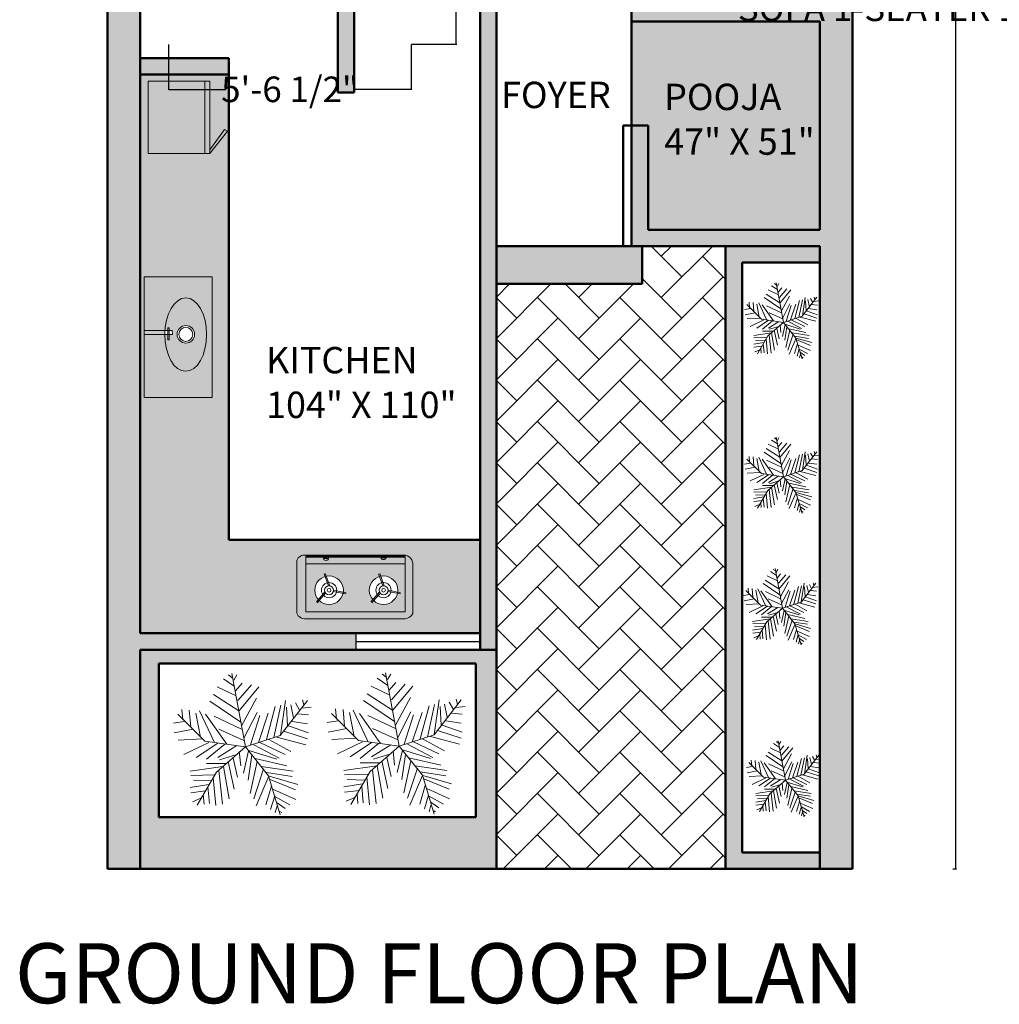
# Model space of a CAD drawing. Units: inches. Extents: x 679 to 1269, y 101 to 755.
# Tile 1 of 6: x 684 to 952, y 101 to 370. Entities that reach past the tile are written whole.
import ezdxf

# ---------------------------------------------------------------- set-up
doc = ezdxf.new("R2010")
doc.units = ezdxf.units.IN
doc.header["$MEASUREMENT"] = 0
for name, color, linetype, lineweight in [('A-ANNO-DIMS', 2, 'Continuous', 18), ('A-ANNO-TEXT', 7, 'Continuous', 25), ('A-AREA-IDEN', 7, 'Continuous', 25), ('A-FLOR-FIXT', 8, 'Continuous', 18), ('A-FLOR-PATT', 8, 'Continuous', 13), ('A-GLAZ', 4, 'Continuous', 25), ('A-WALL', 7, 'Continuous', 50), ('A-WALL-PATT', 8, 'Continuous', 13), ('L-PLNT', 3, 'Continuous', 13)]:
    doc.layers.add(name, color=color, linetype=linetype, lineweight=lineweight)
doc.styles.get("Standard").update_dxf_attribs({"font": 'arial.ttf'})
doc.dimstyles.get("Standard").update_dxf_attribs({"dimtxt": 7, "dimasz": 0.18, "dimexe": 0.18, "dimexo": 0.0625, "dimgap": 0.09, "dimtad": 0, "dimtih": 1, "dimtoh": 1, "dimzin": 0, "dimdsep": 46, "dimlunit": 3, "dimtxsty": 'Standard', "dimcen": 0.09, "dimadec": 0, "dimazin": 0, "dimtfac": 1, "dimtofl": 0, "dimtmove": 0, "dimatfit": 3, "dimfxl": 1, "dimtolj": 1, "dimtzin": 0, "dimarcsym": 0})

# ---------------------------------------------------------------- blocks, each defined once
blk = doc.blocks.new('*D2')
at = {"layer": 'A-ANNO-DIMS', "color": 0, "lineweight": -2, "transparency": 16777216}
for p, q in [((939.6488223970377, 737.729320192004), (940.6166053454735, 737.729320192004)), ((940.4366053454735, 737.5493201920041), (940.4366053454735, 441.3933311060558)), ((940.4366053454737, 137.9093201920038), (940.4366053454735, 434.0653092779521)), ((939.6488223970376, 137.7293201920038), (940.6166053454735, 137.7293201920038))]:
    blk.add_line(p, q, dxfattribs=at)
at = {"layer": 'A-ANNO-DIMS', "color": 0, "transparency": 16777216}
for points in [[(940.4066053454736, 737.5493201920041), (940.4666053454736, 737.5493201920041), (940.4366053454735, 737.729320192004)], [(940.4066053454737, 137.9093201920038), (940.4666053454736, 137.9093201920038), (940.4366053454737, 137.7293201920038)]]:
    blk.add_solid(points, dxfattribs=at)
at = {"layer": 'Defpoints', "color": 0, "transparency": 16777216}
for p in [(939.5863223970377, 737.729320192004), (939.5863223970374, 137.7293201920038), (940.4366053454737, 137.7293201920038)]:
    blk.add_point(p, dxfattribs=at)
at = {"layer": 'A-ANNO-DIMS', "color": 0, "transparency": 16777216, "insert": (940.4366053454735, 437.7293201920036), "char_height": 7, "attachment_point": 5}
blk.add_mtext("\\A1;50'", dxfattribs=at)
blk = doc.blocks.new('*U14')
for p, q in [((-10.18600000000015, 53.63999999999987), (-13.08399999999983, 55.96199999999976)), ((0, 0), (-10.5, 57)), ((-9.098999999999705, 51.7819999999997), (-6.563000000000101, 55.96199999999976)), ((-7.28800000000001, 39.70699999999965), (-21.77800000000025, 46.67299999999977)), ((-8.736999999999625, 47.13799999999969), (-17.06899999999996, 52.71100000000001)), ((-7.65000000000009, 43.42299999999977), (-2.577999999999974, 49.45999999999981)), ((-5.838999999999941, 35.99199999999973), (4.666999999999916, 48.06699999999977)), ((-5.114000000000032, 27.63199999999983), (10.46300000000019, 46.67299999999977)), ((-5.114000000000032, 28.09699999999975), (-24.67599999999993, 40.63599999999996)), ((-3.665000000000418, 19.27299999999968), (-27.57400000000007, 35.52699999999982)), ((-2.940999999999803, 16.48599999999987), (8.652000000000044, 37.84999999999991)), ((16.25900000000001, 5.804999999999836), (23.14199999999983, 31.34799999999973)), ((22.05499999999984, 7.197999999999865), (27.48900000000003, 32.27699999999982)), ((27, 9), (48, 36)), ((27.12699999999995, 9.05600000000004), (31.11200000000008, 35.99199999999973)), ((31.83600000000024, 30.88299999999981), (32.56100000000015, 16.48599999999987)), ((35.09600000000001, 32.74099999999999), (37.26999999999998, 22.52399999999989)), ((38.71900000000005, 34.13399999999979), (41.97899999999981, 28.56099999999992)), ((43.79100000000017, 29.95399999999995), (51.03600000000006, 30.88299999999981)), ((44.15300000000025, 36.45599999999991), (45.23900000000003, 32.74099999999999)), ((-31.5, 4.5), (-52.5, 25.5)), ((-48.58500000000003, 21.13099999999986), (-49.30899999999974, 29.02600000000007)), ((-43.51299999999992, 28.56099999999992), (-42.42699999999968, 15.55799999999976)), ((-38.44199999999955, 26.23899999999981), (-34.81899999999996, 7.662999999999783)), ((-35.54399999999987, 28.09699999999975), (-24.31399999999985, 3.946999999999661)), ((-14.5329999999999, 2.089999999999918), (-30.83399999999983, 25.30999999999995)), ((-24.31399999999985, 23.91699999999969), (-2.940999999999803, 13.69999999999982)), ((-1.128999999999905, 6.733999999999923), (9.014000000000124, 26.70399999999995)), ((3.942000000000007, 1.625), (11.1869999999999, 24.38099999999986)), ((10.10100000000011, 3.482999999999719), (17.70800000000008, 26.23899999999981)), ((40.52999999999975, 25.77499999999986), (48.86200000000008, 24.846)), ((-47.49800000000004, 19.73699999999962), (-55.83000000000038, 18.34399999999982)), ((33.28499999999986, 16.48599999999987), (48.86200000000008, 10.91299999999978)), ((36.18300000000045, 19.73699999999962), (48.13699999999972, 17.87999999999988)), ((-40.61500000000023, 13.69999999999982), (-55.10500000000002, 10.91299999999978)), ((-20.69099999999981, 13.69999999999982), (-1.128999999999905, 4.875999999999976)), ((0, 0), (27, 9)), ((24.22899999999982, 7.662999999999783), (46.6880000000001, 1.625)), ((29.66199999999981, 12.30699999999979), (48.13699999999972, 6.268999999999778)), ((-33.37000000000035, 6.268999999999778), (-52.20699999999988, 5.339999999999918)), ((-28.29899999999998, 3.482999999999719), (-47.86000000000012, -5.805000000000063)), ((-21.41600000000017, 3.017999999999801), (-38.07899999999973, -8.128000000000384)), ((0, 0), (-31.5, 4.5)), ((-15.98199999999951, 2.089999999999918), (-30.11000000000013, -9.521000000000186)), ((0, 0), (-22.5, -19.5)), ((-6.563000000000101, 1.161000000000058), (-21.41600000000017, -8.128000000000384)), ((0, 0), (18, -22.5)), ((6.478000000000065, 1.625), (26.03999999999996, -8.592000000000326)), ((11.1869999999999, 3.482999999999719), (30.74900000000025, -5.805000000000063)), ((18.06999999999971, 5.804999999999836), (35.09600000000001, -3.483000000000174)), ((-6.563000000000101, -5.805000000000063), (-19.96699999999964, -9.985000000000127)), ((-4.751999999999952, -3.483000000000174), (-3.665000000000418, -14.62900000000013)), ((2.493000000000392, -3.019000000000005), (-1.490999999999985, -20.20200000000023)), ((1.769000000000232, -2.555000000000063), (24.22899999999982, -9.521000000000186)), ((5.028999999999996, -6.270000000000209), (2.131000000000312, -25.77500000000009)), ((-17.43100000000004, -15.09400000000005), (-42.78899999999976, -18.80899999999997)), ((-15.2569999999996, -12.77200000000016), (-30.11000000000013, -12.77200000000016)), ((-17.06899999999996, -15.09400000000005), (-12.721, -40.17200000000025)), ((-13.44599999999991, -11.37800000000038), (-8.736999999999625, -32.74100000000021)), ((-9.460999999999785, -8.592000000000326), (-6.201000000000021, -23.4530000000002)), ((9.014000000000124, -11.37800000000038), (3.579999999999927, -35.99200000000019)), ((7.564999999999599, -9.056000000000267), (32.19800000000032, -14.62900000000013)), ((12.27399999999988, -15.09400000000005), (36.9069999999997, -18.80899999999997)), ((-24.31399999999985, -21.59600000000023), (-42.42699999999968, -22.06000000000017)), ((-22.5, -19.5), (-37.5, -45)), ((-20.69099999999981, -18.34500000000003), (-17.79300000000012, -44.35200000000032)), ((14.08499999999958, -16.95100000000025), (6.478000000000065, -40.17200000000025)), ((18.06999999999971, -22.52400000000012), (8.289000000000215, -45.74500000000012)), ((16.25900000000001, -19.73800000000028), (36.18300000000045, -22.98900000000003)), ((18, -22.5), (27, -52.5)), ((18.43300000000045, -22.52400000000012), (40.52999999999975, -29.02600000000007)), ((-28.29899999999998, -29.02600000000007), (-42.78899999999976, -31.34800000000018)), ((-26.8489999999997, -26.24000000000001), (-40.25300000000015, -25.77500000000009)), ((-25.03800000000001, -23.91800000000035), (-22.86500000000024, -45.28100000000017)), ((20.24400000000014, -30.4190000000001), (15.89699999999993, -44.81600000000026)), ((19.1569999999997, -25.31100000000015), (38.71900000000005, -33.20600000000013)), ((-30.83399999999983, -34.13499999999999), (-42.42699999999968, -35.52800000000025)), ((-32.64600000000019, -36.92100000000005), (-31.92099999999982, -44.35200000000032)), ((-29.02300000000014, -30.88400000000002), (-27.93600000000015, -43.88700000000016)), ((22.77999999999975, -37.85000000000014), (19.51900000000023, -48.53200000000015)), ((21.33100000000013, -32.74100000000021), (39.08100000000013, -40.63600000000019)), ((-34.45699999999988, -39.70800000000031), (-40.97800000000006, -42.49400000000014)), ((22.77999999999975, -38.31400000000008), (34.37199999999985, -44.81600000000026)), ((24.59100000000035, -45.74500000000012), (23.14199999999983, -50.85400000000004)), ((24.59100000000035, -43.42300000000022), (30.74900000000025, -47.60300000000029)), ((26.76400000000012, -49.92500000000018), (28.21300000000019, -50.85400000000004))]:
    blk.add_line(p, q)
blk = doc.blocks.new('*D27')
at = {"layer": 'A-ANNO-DIMS', "color": 0, "lineweight": -2, "transparency": 16777216}
for p, q in [((854.1352075964542, 376.6088008284029), (854.1352075964542, 373.1775518326096)), ((876.2268675684088, 376.6088008284029), (876.2268675684088, 373.1775518326096)), ((854.3152075964542, 373.3575518326097), (876.0468675684089, 373.3575518326097)), ((876.2268675684088, 373.3575518326097), (876.4068675684088, 373.3575518326097))]:
    blk.add_line(p, q, dxfattribs=at)
at = {"layer": 'A-ANNO-DIMS', "color": 0, "transparency": 16777216}
for points in [[(854.3152075964542, 373.3875518326096), (854.3152075964542, 373.3275518326097), (854.1352075964542, 373.3575518326097)], [(876.0468675684089, 373.3875518326096), (876.0468675684089, 373.3275518326097), (876.2268675684088, 373.3575518326097)]]:
    blk.add_solid(points, dxfattribs=at)
at = {"layer": 'Defpoints', "color": 0, "transparency": 16777216}
for p in [(854.1352075964542, 376.6713008284029), (876.2268675684088, 376.6713008284029), (876.2268675684088, 373.3575518326097)]:
    blk.add_point(p, dxfattribs=at)
at = {"layer": 'A-ANNO-DIMS', "color": 0, "transparency": 16777216, "insert": (940.4733341441251, 373.3575518326097), "char_height": 7, "attachment_point": 5}
blk.add_mtext('\\A1;SOFA 1-SEATER 1\'-10" TYP.', dxfattribs=at)
blk = doc.blocks.new('*D49')
at = {"layer": 'A-ANNO-DIMS', "color": 0, "lineweight": -2, "transparency": 16777216}
for p, q in [((791.4614275537712, 445.6571882207567), (803.9031303932073, 445.6571882207567)), ((803.7231303932074, 445.4771882207567), (803.7231303932074, 408.2858845313227)), ((803.7231303932074, 363.6758359578504), (803.7231303932074, 400.8671396472845)), ((791.4614275537712, 363.4958359578504), (803.9031303932073, 363.4958359578504))]:
    blk.add_line(p, q, dxfattribs=at)
at = {"layer": 'A-ANNO-DIMS', "color": 0, "transparency": 16777216}
for points in [[(803.6931303932075, 445.4771882207567), (803.7531303932075, 445.4771882207567), (803.7231303932074, 445.6571882207567)], [(803.6931303932075, 363.6758359578504), (803.7531303932075, 363.6758359578504), (803.7231303932074, 363.4958359578504)]]:
    blk.add_solid(points, dxfattribs=at)
at = {"layer": 'Defpoints', "color": 0, "transparency": 16777216}
for p in [(791.398927553771, 445.6571882207567), (791.398927553771, 363.4958359578504), (803.7231303932074, 363.4958359578504)]:
    blk.add_point(p, dxfattribs=at)
at = {"layer": 'A-ANNO-DIMS', "color": 0, "transparency": 16777216, "insert": (803.7231303932074, 404.5765120893032), "char_height": 7, "attachment_point": 5}
blk.add_mtext('\\A1;KITCHEN SINK 6\'-10"', dxfattribs=at)
blk = doc.blocks.new('*D50')
at = {"layer": 'A-ANNO-DIMS', "color": 0, "lineweight": -2, "transparency": 16777216}
for p, q in [((724.8937546393688, 363.4333359578503), (724.8937546393688, 350.9916331184144)), ((791.3989275537707, 363.4333359578503), (791.3989275537707, 350.9916331184144)), ((725.0737546393686, 351.1716331184144), (740.5969277268562, 351.1716331184144)), ((791.2189275537708, 351.1716331184144), (775.6957544662833, 351.1716331184144))]:
    blk.add_line(p, q, dxfattribs=at)
at = {"layer": 'A-ANNO-DIMS', "color": 0, "transparency": 16777216}
for points in [[(725.0737546393686, 351.2016331184144), (725.0737546393686, 351.1416331184144), (724.8937546393688, 351.1716331184144)], [(791.2189275537708, 351.2016331184144), (791.2189275537708, 351.1416331184144), (791.3989275537707, 351.1716331184144)]]:
    blk.add_solid(points, dxfattribs=at)
at = {"layer": 'Defpoints', "color": 0, "transparency": 16777216}
for p in [(724.8937546393688, 363.4958359578503), (791.3989275537707, 363.4958359578503), (724.8937546393688, 351.1716331184144)]:
    blk.add_point(p, dxfattribs=at)
at = {"layer": 'A-ANNO-DIMS', "color": 0, "transparency": 16777216, "insert": (758.1463410965698, 351.1716331184144), "char_height": 7, "attachment_point": 5}
blk.add_mtext('\\A1;5\'-6 1/2"', dxfattribs=at)

msp = doc.modelspace()

# ---------------------------------------------------------------- hatches: boundary and pattern name
at = {"layer": 'A-FLOR-FIXT'}
h = msp.add_hatch(color=256, dxfattribs=at)
h.dxf.hatch_style = 1
h.paths.add_polyline_path([(718.0629616280667, 350.2339561763691), (719.3848963068058, 350.2339561763691), (719.3848963068058, 337.3636525715756), (718.0629616280667, 337.3636525715756)])
at = {"layer": 'A-FLOR-PATT'}
h = msp.add_hatch(dxfattribs=at)
h.set_pattern_fill('ANSI31', color=256)
h.set_pattern_definition([(45, (0, 0), (-0.0883883476483185, 0.0883883476483185), [])])
h.paths.add_polyline_path([(1119.80525126775, 251.5418490076826), (1104.538824747302, 251.5418490076827), (1104.538824747302, 181.2270478723494), (1119.805251267749, 181.2270478723494)])
h.paths.add_polyline_path([(1111.467825253477, 194.1386832997395), (1110.456531068886, 194.1386832997395), (1110.456531068886, 207.2855076986381), (1109.186667875484, 207.2855076986381, -0.4142135623730952), (1108.433942699824, 208.0382328742978), (1108.433942699824, 222.7134894754692, -0.4142135623730952), (1109.186667875484, 223.4662146511288), (1110.456531068886, 223.4662146511288), (1110.456531068886, 236.6130390500275), (1111.467825253365, 236.6130390500275, -0.0640418572951994), (1112.984766530213, 234.1937808082358), (1112.984766530213, 223.4662146511288), (1113.243335539084, 223.4662146511288, -0.4142135623730992), (1113.996060714743, 222.7134894754692), (1113.996060714743, 208.0382328742978, -0.4142135623730951), (1113.243335539084, 207.2855076986381), (1112.984766530213, 207.2855076986381), (1112.984766530213, 196.557941541411, -0.0640418572915539)], flags=16)
h.paths.add_polyline_path([(794.4135080734268, 488.8112779029178), (775.7855460058269, 488.8112779029178), (775.7855460058269, 449.7293201920038), (775.785546005827, 418.4964767675847), (794.4135080734268, 418.4964767675847)])
h.paths.add_polyline_path([(785.1342662046906, 431.4081121949747), (784.1229720201133, 431.4081121949747, -0.0640418572917201), (782.6060307433639, 433.8273704366466), (782.6060307433639, 444.5549365938734), (782.3474617344928, 444.5549365938734, -0.4142135623730399), (781.5947365588333, 445.307661769533), (781.5947365588332, 459.9829183707044, -0.414213562373073), (782.3474617344928, 460.7356435463641), (782.6060307433639, 460.7356435463641), (782.6060307433639, 471.4632097034709, -0.0640418572952049), (784.1229720202114, 473.8824679452628), (785.1342662046906, 473.8824679452628), (785.1342662046906, 460.7356435463641), (786.4041293980922, 460.7356435463641, -0.414213562373073), (787.1568545737518, 459.9829183707044), (787.1568545737518, 445.307661769533, -0.4142135623730951), (786.4041293980922, 444.5549365938734), (785.1342662046906, 444.5549365938734)], flags=16)
h = msp.add_hatch(dxfattribs=at)
h.set_pattern_fill('AR-HBONE', color=256, scale=2)
h.set_pattern_definition([(45, (0, 0), (0, 11.31370849898476), [24, -8]), (135, (5.65685425, 5.65685425), (9e-16, 11.31370849898476), [24, -8])])
h.paths.add_polyline_path([(877.4640921397338, 308.2293201920038), (854.5894706319959, 308.2293201920038), (854.5894706319959, 297.8792233000386), (814.714092139734, 297.8792233000386), (814.714092139734, 137.7293201920038), (877.4640921397338, 137.7293201920038)])
at = {"layer": 'A-WALL-PATT'}
h = msp.add_hatch(color=256, dxfattribs=at)
h.dxf.hatch_style = 1
h.paths.add_polyline_path([(775.785546005827, 535.7293201920038), (771.2855460058269, 535.7293201920038), (771.2855460058269, 454.2293201920037), (717.2140921397341, 454.2293201920037), (717.2140921397341, 531.2293201920038), (742.5592373165279, 531.2293201920038), (742.5592373165279, 535.7293201920038), (717.214092139734, 535.7293201920038), (717.214092139734, 583.7293201920037), (775.7855460058269, 583.7293201920037), (775.7855460058269, 588.8832314657213), (775.7855460058269, 623.2426399571717), (775.7855460058269, 645.3287176756929), (771.285546005827, 645.3287176756929), (771.285546005827, 588.2293201920039), (717.214092139734, 588.2293201920037), (717.214092139734, 674.2293201920038), (734.5886313004448, 674.2293201920039), (734.5886313004448, 678.7293201920038), (717.214092139734, 678.7293201920038), (717.214092139734, 728.7293201920038), (903.214092139734, 728.7293201920037), (903.2140921397338, 588.2293201920041), (810.214092139734, 588.2293201920039), (810.214092139734, 583.7293201920037), (903.2140921397338, 583.7293201920037), (903.214092139734, 374.2293201920038), (851.714092139734, 374.2293201920038), (851.7140921397341, 369.7293201920038), (903.214092139734, 369.7293201920038), (903.214092139734, 312.7293201920038), (856.2140921397341, 312.7293201920038), (856.2140921397341, 341.2293201920037), (851.7140921397341, 341.2293201920038), (851.714092139734, 308.2293201920038), (903.214092139734, 308.2293201920038), (903.214092139734, 137.7293201920038), (912.214092139734, 137.7293201920038), (912.214092139734, 737.7293201920037), (708.214092139734, 737.7293201920037), (708.214092139734, 137.7293201920039), (717.214092139734, 137.729320192004), (717.214092139734, 197.7631775657537), (776.1957429582106, 197.7631775657537), (776.1957429582106, 202.2631775657537), (717.214092139734, 202.2631775657538), (717.2140921397341, 449.7293201920038), (771.2855460058272, 449.7293201920037), (771.285546005827, 350.2976097466271), (775.7855460058273, 350.2976097466273), (775.7855460058272, 531.2293201920038)])
h = msp.add_hatch(color=256, dxfattribs=at)
h.dxf.hatch_style = 1
h.paths.add_polyline_path([(810.2140921397339, 227.8284629457475), (741.4953169629443, 227.8284629457476), (741.4953169629443, 355.2293201920037), (717.2140921397341, 355.2293201920038), (717.214092139734, 202.2631775657537), (810.2140921397339, 202.2631775657537)])
h.paths.add_polyline_path([(760.0690219295593, 222.2577028080951, -0.3244181347622923), (762.5160615469127, 223.6639245446819), (788.7526899728937, 223.6639245446819, -0.4472035247863912), (791.8294020877602, 221.2701314030444), (791.8294020877602, 207.6479060594974, -0.261429945449989), (789.6882560863445, 206.2452345624028), (762.5160615388623, 206.2452345617986, -0.3295456964687033), (760.0690219295593, 207.7222576236091)], flags=16)
h.paths.add_polyline_path([(762.5160615393341, 221.2701313990216), (789.6882560854228, 221.2701313990216), (789.6882560854228, 208.129714781982), (762.5160615393341, 208.129714781982)], flags=0)
edge = h.paths.add_edge_path(flags=0)
edge.add_ellipse((783.812830230725, 223.042858951823), major_axis=(0.7131854232762685, -0.0201982968358234), ratio=0.3769733725084229, start_angle=41.86570148012203, end_angle=148.308268672003, ccw=False)
edge.add_line((783.8793567947503, 223.3091220170284), (790.0170442706001, 223.2828463353598))
edge.add_line((790.0170442706001, 223.2828463353598), (784.0963805280572, 223.2828463353598))
edge.add_ellipse((783.812830230725, 223.042858951823), major_axis=(0.7131854232762685, -0.0201982968358234), ratio=0.3769733725084229, start_angle=346.43382291563427, end_angle=401.86570148012197, ccw=False)
edge.add_ellipse((783.8052160111637, 222.7740070373799), major_axis=(0.6638606992674089, -0.0428711540118445), ratio=0.4928397098496223, start_angle=169.7196154411588, end_angle=373.72857998462126, ccw=False)
edge.add_ellipse((783.812830230725, 223.042858951823), major_axis=(0.7131854232762685, -0.0201982968358234), ratio=0.3769733725084229, start_angle=148.308268672003, end_angle=192.1304824464817, ccw=False)
h.paths.add_polyline_path([(772.8079330483064, 214.0382508827421, -1), (764.9837244191427, 214.0382508827421, -1)], flags=0)
h.paths.add_polyline_path([(766.8162108612969, 214.0382508827421, -1), (770.9754466061521, 214.0382508827421, -1)], flags=0)
h.paths.add_polyline_path([(767.6711011316813, 214.0382508827421, -1), (770.1205563357677, 214.0382508827421, -1)], flags=0)
edge = h.paths.add_edge_path(flags=0)
edge.add_ellipse((768.035203354937, 222.5467921924825), major_axis=(0.6638606992674086, -0.0428711540118445), ratio=0.4928397098496223, start_angle=165.080460978896, end_angle=377.669946342211, ccw=False)
edge.add_ellipse((768.0563319620411, 222.87396910689), major_axis=(0.7131854232762685, -0.0201982968358234), ratio=0.3769733725084229, start_angle=342.91013703044274, end_angle=554.300550688774, ccw=False)
h.paths.add_polyline_path([(769.4027141166019, 214.0382508827421, -1), (768.3889433508471, 214.0382508827421, -1)], flags=0)
h.paths.add_polyline_path([(787.7210304354861, 214.0382508827421, -1), (779.8968218063224, 214.0382508827421, -1)], flags=0)
h.paths.add_polyline_path([(781.7293082484767, 214.0382508827421, -1), (785.8885439933318, 214.0382508827421, -1)], flags=0)
h.paths.add_polyline_path([(782.5841985188611, 214.0382508827421, -1), (785.0336537229475, 214.0382508827421, -1)], flags=0)
h.paths.add_polyline_path([(718.2843006566472, 266.7946890571272), (718.2843006566472, 299.8104473136175), (736.8525415124183, 299.8104473136175), (736.8525415124183, 266.7946890571272)], flags=16)
h.paths.add_polyline_path([(784.3158115037817, 214.0382508827421, -1), (783.3020407380269, 214.0382508827421, -1)], flags=0)
edge = h.paths.add_edge_path(flags=0)
edge.add_ellipse((729.6517749280199, 284.0271019961246), major_axis=(0.0276881913638295, 10.06083745494668), ratio=0.5689904069289867, start_angle=89.77278696833508, end_angle=78.68100194365502, ccw=False)
edge.add_ellipse((729.6517749280199, 284.0271019961246), major_axis=(0.0276881913638295, 10.06083745494668), ratio=0.5689904069289867, start_angle=78.68100194365502, end_angle=89.77278696833508, ccw=False)
h.paths.add_polyline_path([(727.2953260935, 284.083274375772, -1), (732.089020927023, 284.083274375772, -1)], flags=0)
h.paths.add_polyline_path([(727.7783840642574, 284.083274375772, -1), (731.6059629562654, 284.083274375772, -1)], flags=0)
h.paths.add_polyline_path([(725.1513430178541, 282.6112946821611), (724.789534887559, 282.6041909271886), (724.7738237451905, 285.8924188729091), (725.135657556808, 285.8941477136776), (725.1390638223173, 285.1812410913929), (725.9788456803889, 285.1812410913929), (725.9841764125675, 284.065557577768), (725.1443945544959, 284.065557577768)], flags=0)
h.paths.add_polyline_path([(719.3848963068058, 333.5705183253991), (719.3848963068058, 353.3971975653831), (736.2214701214579, 353.3971975653831), (736.2214701214579, 334.653021312364), (740.2779245480251, 340.16267501584), (741.0502032336526, 339.7071400477636), (736.2214701214579, 333.5705183253991)], flags=16)
h.paths.add_polyline_path([(751.547841028177, 418.1612455991298), (736.9517971173841, 418.1612455991298), (717.2140921397341, 400.0134649693153), (771.2855460058272, 400.0134649693153)])
h.paths.add_polyline_path([(736.9517971173841, 418.1612455991298), (726.7684779999342, 418.1612455991298, -0.4142135623730951), (724.8937546393689, 420.0359689596953), (724.8937546393688, 442.6682748216227), (717.2140921397341, 449.7293201920038), (717.2140921397341, 400.0134649693153)])
h.paths.add_polyline_path([(771.2855460058272, 449.7293201920038), (765.8691621322733, 444.7492403673522, -0.1362876450951072), (766.1376685718088, 443.782464860191), (766.137668571809, 420.0359689596953, -0.4142135623730951), (764.2629452112434, 418.1612455991298), (751.547841028177, 418.1612455991298), (771.2855460058272, 400.0134649693153)])
h.paths.add_polyline_path([(771.285546005827, 449.7293201920037), (717.2140921397341, 449.7293201920038), (724.8937546393688, 442.6682748216227), (724.8937546393689, 443.782464860191, -0.4142135623730951), (726.7684779999342, 445.6571882207565), (764.2629452112434, 445.6571882207565, -0.2630747701129512), (765.8691621322733, 444.7492403673522)])
h.paths.add_polyline_path([(797.165656172381, 526.2156153371322), (807.610883585287, 526.2156153371322), (807.610883585287, 532.4386050637592), (797.165656172381, 532.4386050637592)], flags=9)
h.paths.add_polyline_path([(795.5756520696247, 567.5889172437371), (805.736472721491, 567.5889172437371), (805.736472721491, 573.918028896125), (795.5756520696247, 573.918028896125)], flags=9)
h.paths.add_polyline_path([(858.7905219185442, 331.2865523050099), (904.3639982061288, 331.2865523050099), (904.3639982061288, 342.3348914147287), (858.7905219185442, 342.3348914147287)], flags=9)
h.paths.add_polyline_path([(858.7659208517223, 343.5022493445522), (896.6687845042359, 343.5022493445522), (896.6687845042359, 354.6981948552025), (858.7659208517223, 354.6981948552025)], flags=9)
h.paths.add_polyline_path([(797.3091566163783, 428.2611229613246), (854.0933390547062, 428.2611229613246), (854.0933390547062, 439.31684239109), (797.3091566163783, 439.31684239109)], flags=9)
h.paths.add_polyline_path([(797.2870156562387, 440.4842003209135), (877.7226637371487, 440.4842003209135), (877.7226637371487, 451.6727655115172), (797.2870156562387, 451.6727655115172)], flags=9)
h.paths.add_polyline_path([(715.5521415298247, 369.6252991971824), (756.6845864844926, 369.6252991971824), (756.6845864844926, 379.5970028566379), (715.5521415298247, 379.5970028566379)], flags=9)
h.paths.add_polyline_path([(715.5310479683095, 380.6517146058336), (773.4872735125329, 380.6517146058336), (773.4872735125329, 390.7499796343803), (715.5310479683095, 390.7499796343803)], flags=9)
h.paths.add_polyline_path([(814.121643488478, 344.0476457953973), (852.5657306110735, 344.0476457953973), (852.5657306110735, 355.2435913060476), (814.121643488478, 355.2435913060476)], flags=9)
h.paths.add_polyline_path([(749.8011169905323, 259.2218704960809), (806.582839322178, 259.2218704960809), (806.582839322178, 270.2702096057997), (749.8011169905323, 270.2702096057997)], flags=25)
h.paths.add_polyline_path([(749.7777459770516, 271.4387975889643), (797.7350656396789, 271.4387975889643), (797.7350656396789, 282.627362779568), (749.7777459770516, 282.627362779568)], flags=25)
h.paths.add_polyline_path([(730.2802183090811, 479.0995485901093), (762.9437350181166, 479.0995485901093), (762.9437350181166, 487.0181371752795), (730.2802183090811, 487.0181371752795)], flags=9)
h.paths.add_polyline_path([(730.262586181303, 487.854808378626), (771.0580402216244, 487.854808378626), (771.0580402216244, 495.8791897304651), (730.262586181303, 495.8791897304651)], flags=9)
h = msp.add_hatch(color=256, dxfattribs=at)
h.dxf.hatch_style = 1
h.paths.add_polyline_path([(903.214092139734, 511.7293201920038), (810.214092139734, 511.7293201920038), (810.214092139734, 507.2293201920038), (903.214092139734, 507.2293201920038)])
h.paths.add_polyline_path([(881.9640921397338, 303.7293201920038), (903.214092139734, 303.7293201920038), (903.214092139734, 308.2293201920038), (877.4640921397338, 308.2293201920038), (877.4640921397338, 137.7293201920038), (903.2140921397338, 137.7293201920038), (903.2140921397338, 142.2293201920038), (881.9640921397338, 142.2293201920039), (881.9640921397338, 151.2293201920038)])
h.paths.add_polyline_path([(814.714092139734, 379.5403287480949), (810.214092139734, 379.5403287480949), (810.2140921397339, 197.7631775657538), (814.714092139734, 197.7631775657537)])
h = msp.add_hatch(color=256, dxfattribs=at)
h.dxf.hatch_style = 1
h.paths.add_polyline_path([(903.214092139734, 369.7293201920038), (851.7140921397338, 369.7293201920038), (851.7140921397338, 341.2293201920038), (856.2140921397341, 341.2293201920038), (856.2140921397341, 312.7293201920038), (903.214092139734, 312.7293201920038)])
h = msp.add_hatch(color=256, dxfattribs=at)
h.dxf.hatch_style = 1
h.paths.add_polyline_path([(741.4953169629443, 359.7293201920038), (717.2140921397341, 359.7293201920038), (717.214092139734, 355.2293201920039), (741.4953169629443, 355.2293201920038)])
h = msp.add_hatch(color=256, dxfattribs=at)
h.dxf.hatch_style = 1
h.paths.add_polyline_path([(734.8739277227982, 353.3971975653831), (719.3848963068058, 353.3971975653831), (719.3848963068058, 333.5705183253991), (734.8739277227982, 333.5705183253991)])
h.paths.add_polyline_path([(736.2214701214579, 353.3971975653831), (734.8739277227982, 353.3971975653831), (734.8739277227982, 333.5705183253991), (736.2214701214579, 333.5705183253991)])
h.paths.add_polyline_path([(741.0502032336526, 339.7071400477636), (740.2779245480251, 340.16267501584), (736.2214701214579, 334.653021312364), (736.2214701214579, 333.5705183253991)])
edge = h.paths.add_edge_path()
edge.add_line((736.8525415124183, 299.8104473136175), (718.2843006566472, 299.8104473136175))
edge.add_line((718.2843006566472, 299.8104473136175), (718.2843006566472, 285.1812410913929))
edge.add_line((718.2843006566472, 285.1812410913929), (723.9671580958066, 285.1812410913929))
edge.add_ellipse((729.6517749280199, 284.0271019961246), major_axis=(0.0276881913638295, 10.06083745494668), ratio=0.5689904069289867, start_angle=89.77278696833508, end_angle=78.68100194365502, ccw=False)
edge.add_line((723.9273319790111, 284.065557577768), (718.2843006566472, 284.065557577768))
edge.add_line((718.2843006566472, 284.065557577768), (718.2843006566472, 266.7946890571272))
edge.add_line((718.2843006566472, 266.7946890571272), (736.8525415124183, 266.7946890571272))
edge.add_line((736.8525415124183, 266.7946890571272), (736.8525415124183, 299.8104473136175))
edge = h.paths.add_edge_path(flags=17)
edge.add_ellipse((729.6517749280199, 284.0271019961246), major_axis=(0.0276881913638295, 10.06083745494668), ratio=0.5689904069289867, start_angle=-270.227213031665, end_angle=78.68100194365502)
edge.add_line((723.9671580958066, 285.1812410913929), (724.7772217503043, 285.1812410913929))
edge.add_line((724.7772217503043, 285.1812410913929), (724.7738237451905, 285.8924188729091))
edge.add_line((724.7738237451905, 285.8924188729091), (725.135657556808, 285.8941477136776))
edge.add_line((725.135657556808, 285.8941477136776), (725.1390638223173, 285.1812410913929))
edge.add_line((725.1390638223173, 285.1812410913929), (725.9788456803889, 285.1812410913929))
edge.add_line((725.9788456803889, 285.1812410913929), (725.9841764125675, 284.065557577768))
edge.add_line((725.9841764125675, 284.065557577768), (725.1443945544959, 284.065557577768))
edge.add_line((725.1443945544959, 284.065557577768), (725.1513430178541, 282.6112946821611))
edge.add_line((725.1513430178541, 282.6112946821611), (724.789534887559, 282.6041909271886))
edge.add_line((724.789534887559, 282.6041909271886), (724.7825524824829, 284.065557577768))
edge.add_line((724.7825524824829, 284.065557577768), (723.9273319790111, 284.065557577768))
h.paths.add_polyline_path([(732.089020927023, 284.083274375772, -1), (727.2953260935, 284.083274375772, -1)], flags=16)
h.paths.add_polyline_path([(731.6059629562654, 284.083274375772, -1), (727.7783840642574, 284.083274375772, -1)], flags=0)
edge = h.paths.add_edge_path(flags=17)
edge.add_ellipse((729.6517749280199, 284.0271019961246), major_axis=(0.0276881913638295, 10.06083745494668), ratio=0.5689904069289867, start_angle=78.68100194365502, end_angle=89.77278696833508, ccw=False)
edge.add_line((723.9671580958066, 285.1812410913929), (718.2843006566472, 285.1812410913929))
edge.add_line((718.2843006566472, 285.1812410913929), (718.2843006566472, 284.065557577768))
edge.add_line((718.2843006566472, 284.065557577768), (723.9273319790111, 284.065557577768))
h = msp.add_hatch(color=256, dxfattribs=at)
h.dxf.hatch_style = 1
h.paths.add_polyline_path([(854.5894706319959, 308.2293201920038), (851.7140921397338, 308.2293201920038), (814.714092139734, 308.2293201920038), (814.714092139734, 297.8792233000386), (854.5894706319959, 297.8792233000386)])
h.paths.add_polyline_path([(814.714092139734, 197.7631775657538), (717.214092139734, 197.7631775657537), (717.214092139734, 137.7293201920038), (814.714092139734, 137.7293201920038)])
h.paths.add_polyline_path([(722.2438019341816, 151.8883412274699), (722.2438019341816, 194.0207146279499), (809.1022054683272, 194.0207146279499), (809.1022054683272, 151.8883412274699)], flags=16)
h = msp.add_hatch(color=256, dxfattribs=at)
h.dxf.hatch_style = 1
h.paths.add_polyline_path([(791.8294020877602, 221.2701314030444, 0.4472035247863919), (788.7526899728937, 223.6639245446819), (762.5160615469127, 223.6639245446819, 0.3244181347622925), (760.0690219295593, 222.2577028080951), (760.0690219295593, 207.7222576236091, 0.3295456964687013), (762.5160615388623, 206.2452345617986), (789.6882560863445, 206.2452345624028, 0.2614299454499895), (791.8294020877602, 207.6479060594974)])
h.paths.add_polyline_path([(787.7210304354861, 214.0382508827421, -1), (779.8968218063224, 214.0382508827421, -1)], flags=16)
h.paths.add_polyline_path([(785.8885439933318, 214.0382508827421, -1), (781.7293082484767, 214.0382508827421, -1)], flags=0)
h.paths.add_polyline_path([(785.0336537229475, 214.0382508827421, -1), (782.5841985188611, 214.0382508827421, -1)], flags=0)
edge = h.paths.add_edge_path(flags=16)
edge.add_ellipse((783.812830230725, 223.042858951823), major_axis=(0.7131854232762685, -0.0201982968358234), ratio=0.3769733725084229, start_angle=41.86570148013669, end_angle=148.3082686719917, ccw=False)
edge.add_ellipse((783.812830230725, 223.042858951823), major_axis=(0.7131854232762685, -0.0201982968358234), ratio=0.3769733725084229, start_angle=346.4338229157989, end_angle=401.8657014801367, ccw=False)
edge.add_ellipse((783.8052160111637, 222.7740070373799), major_axis=(0.6638606992674089, -0.0428711540118445), ratio=0.4928397098496223, start_angle=169.7196154411588, end_angle=373.72857998463945, ccw=False)
edge.add_ellipse((783.812830230725, 223.042858951823), major_axis=(0.7131854232762685, -0.0201982968358234), ratio=0.3769733725084229, start_angle=148.3082686719917, end_angle=192.1304824464878, ccw=False)
h.paths.add_polyline_path([(772.8079330483064, 214.0382508827421, -1), (764.9837244191427, 214.0382508827421, -1)], flags=16)
h.paths.add_polyline_path([(766.8162108612969, 214.0382508827421, -1), (770.9754466061521, 214.0382508827421, -1)], flags=0)
h.paths.add_polyline_path([(767.6711011316813, 214.0382508827421, -1), (770.1205563357677, 214.0382508827421, -1)], flags=0)
h.paths.add_polyline_path([(784.3158115037817, 214.0382508827421, -1), (783.3020407380269, 214.0382508827421, -1)], flags=0)
h.paths.add_polyline_path([(769.4027141166019, 214.0382508827421, -1), (768.3889433508471, 214.0382508827421, -1)], flags=0)
edge = h.paths.add_edge_path(flags=16)
edge.add_ellipse((768.035203354937, 222.5467921924825), major_axis=(0.6638606992674086, -0.0428711540118445), ratio=0.4928397098496223, start_angle=165.0804609789027, end_angle=377.6699463424078, ccw=False)
edge.add_ellipse((768.0563319620411, 222.87396910689), major_axis=(0.7131854232762685, -0.0201982968358234), ratio=0.3769733725084229, start_angle=342.9101370313131, end_angle=554.300550688774, ccw=False)

# ---------------------------------------------------------------- linework, layer by layer
at = {"layer": 'A-FLOR-FIXT'}
for p, q in [((736.2214701214579, 353.3971975653831), (719.3848963068058, 353.3971975653831)), ((719.3848963068058, 353.3971975653831), (719.3848963068058, 333.5705183253991)), ((734.8739277227982, 333.5705183253991), (734.8739277227982, 353.3971975653831)), ((736.2214701214579, 333.5705183253991), (736.2214701214579, 353.3971975653831)), ((740.2779245480251, 340.16267501584), (736.2214701214579, 334.653021312364)), ((736.2214701214579, 333.5705183253991), (741.0502032336526, 339.7071400477636)), ((741.0502032336526, 339.7071400477636), (740.2779245480251, 340.16267501584)), ((719.3848963068058, 333.5705183253991), (736.2214701214579, 333.5705183253991)), ((718.2843006566472, 299.8104473136175), (736.8525415124183, 299.8104473136175)), ((718.2843006566472, 266.7946890571272), (718.2843006566472, 299.8104473136175)), ((736.8525415124183, 299.8104473136175), (736.8525415124183, 266.7946890571272)), ((724.7738237451905, 285.8924188729091), (725.135657556808, 285.8941477136776)), ((724.789534887559, 282.6041909271886), (724.7738237451905, 285.8924188729091)), ((725.135657556808, 285.8941477136776), (725.1513430178541, 282.6112946821611)), ((725.9788456803889, 285.1812410913929), (718.2843006566472, 285.1812410913929)), ((725.9841764125675, 284.065557577768), (718.2843006566472, 284.065557577768)), ((725.9841764125675, 284.065557577768), (725.9788456803889, 285.1812410913929)), ((724.789534887559, 282.6041909271886), (725.1513430178541, 282.6112946821611)), ((736.8525415124183, 266.7946890571272), (718.2843006566472, 266.7946890571272)), ((760.0690219295593, 207.7222576258752), (760.0690219295593, 222.2577028070624)), ((788.7526899748864, 223.6639245446819), (762.5160615393341, 223.6639245446819)), ((762.5160615393343, 223.2828463353598), (789.688256085423, 223.2828463353598)), ((762.5160615393343, 223.2828463353598), (762.5160615393341, 208.129714781982)), ((789.6882560854228, 221.2701313990216), (762.5160615393341, 221.2701313990216)), ((789.6882560854228, 208.129714781982), (789.6882560854228, 223.2828463353598)), ((791.8294020877602, 207.6479060585658), (791.8294020877602, 221.2701313990216)), ((768.691765655336, 215.2458584174561), (767.555305764583, 218.5664088699083)), ((769.0644607362719, 215.2513135137084), (767.8462860421658, 218.6526368969168)), ((783.6048630443784, 215.2458584174561), (782.4684031517627, 218.5664088699083)), ((783.9775581234516, 215.2513135137084), (782.7593834293456, 218.6526368969168)), ((767.7609696784438, 213.5777591640177), (765.424424568695, 210.8221272417392)), ((767.9520414700182, 213.2577233050066), (765.6445903689983, 210.6132449420217)), ((769.9458955978425, 213.7127599274787), (773.5006153998347, 213.0670684674802)), ((770.1275188853415, 214.0382508827421), (773.5714298771145, 213.3621787937406)), ((782.6740670656236, 213.5777591640177), (780.3375219558748, 210.8221272417392)), ((782.8651388571978, 213.2577233050066), (780.5576877580406, 210.6132449420217)), ((784.8589929850223, 213.7127599274787), (788.4137127870144, 213.0670684674802)), ((785.0406162725212, 214.0382508827421), (788.4845272642942, 213.3621787937406)), ((762.5160615393341, 208.129714781982), (789.6882560854228, 208.129714781982)), ((789.6882560863462, 206.2452345624028), (762.5160615388631, 206.2452345617986))]:
    msp.add_line(p, q, dxfattribs=at)
for centre, radius in [((729.6921735102615, 284.083274375772), 2.396847416761485), ((729.6921735102615, 284.083274375772), 1.913789446004076), ((768.8958287337246, 214.0382508827421), 3.912104314581809), ((768.8958287337246, 214.0382508827421), 2.07961787242757), ((783.8089261209042, 214.0382508827421), 3.912104314581809), ((783.8089261209042, 214.0382508827421), 2.07961787242757), ((768.8958287337246, 214.0382508827421), 1.224727602043285), ((768.8958287337246, 214.0382508827421), 0.5068853828773451), ((783.8089261209042, 214.0382508827421), 1.224727602043285), ((783.8089261209042, 214.0382508827421), 0.5068853828773451)]:
    msp.add_circle(centre, radius, dxfattribs=at)
for centre, radius, start, end in [((762.2621399243744, 221.2735654191162), 2.403808008050551, 83.93635847429258, 156.894011911223), ((789.2204730310859, 221.0910340087536), 2.61506915767081, 3.927071439933448, 100.3045183047211), ((762.291354517025, 208.6385167628574), 2.403808008050551, 202.4061646789659, 275.3638181333238), ((789.5091586956205, 208.8541636193219), 2.61506915767081, 273.9270714417616, 332.5307974806221)]:
    msp.add_arc(centre, radius, start, end, dxfattribs=at)
at = {"layer": 'A-FLOR-FIXT', "extrusion": (0, 0, -0.9999999999999998)}
msp.add_ellipse((729.6517749280199, 284.0271019961246), major_axis=(0.0276881913638295, 10.06083745494667), ratio=0.5689904069289868, dxfattribs=at)
at = {"layer": 'A-FLOR-FIXT'}
for centre, major_axis, ratio in [((768.0563319620411, 222.87396910689), (0.7131854232762685, -0.0201982968358234), 0.376973372508423), ((768.035203354937, 222.5467921924825), (0.6638606992674086, -0.0428711540118445), 0.4928397098496223), ((783.812830230725, 223.042858951823), (0.7131854232762685, -0.0201982968358234), 0.376973372508423), ((783.8052160111637, 222.7740070373799), (0.6638606992674086, -0.0428711540118445), 0.4928397098496223)]:
    msp.add_ellipse(centre, major_axis=major_axis, ratio=ratio, dxfattribs=at)
at = {"layer": 'A-GLAZ'}
for p, q in [((776.1957429582106, 202.2631775657537), (776.1957429582106, 197.7631775657537)), ((810.2140921397339, 202.2631775657537), (776.1957429582106, 202.2631775657537)), ((776.1957429582106, 202.2631775657537), (776.1957429582106, 200.0131775657537)), ((810.2140921397339, 197.7631775657538), (810.2140921397339, 202.2631775657537)), ((776.1957429582106, 200.0131775657537), (810.2140921397339, 200.0131775657537)), ((776.1957429582106, 197.7631775657537), (810.2140921397339, 197.7631775657538))]:
    msp.add_line(p, q, dxfattribs=at)
at = {"layer": 'A-WALL'}
for p, q in [((708.214092139734, 137.7293201920038), (708.214092139734, 737.7293201920037)), ((912.214092139734, 737.7293201920037), (912.214092139734, 137.7293201920038)), ((775.7855460058273, 350.2976097466273), (775.7855460058272, 531.2293201920038)), ((717.214092139734, 202.2631775657537), (717.2140921397341, 449.7293201920038)), ((771.285546005827, 350.2976097466271), (771.2855460058272, 449.7293201920036)), ((810.2140921397339, 197.7631775657537), (810.214092139734, 379.5403287480949)), ((814.714092139734, 137.7293201920038), (814.714092139734, 379.5403287480949)), ((851.714092139734, 374.2293201920039), (851.7140921397341, 369.7293201920038)), ((851.7140921397338, 369.7293201920038), (903.2140921397342, 369.7293201920038)), ((851.7140921397338, 369.7293201920038), (851.7140921397338, 341.2293201920038)), ((903.214092139734, 369.7293201920038), (903.214092139734, 312.7293201920038)), ((717.2140921397339, 359.7293201920038), (741.4953169629443, 359.7293201920038)), ((741.4953169629443, 359.7293201920038), (741.4953169629443, 355.2293201920038)), ((717.2140921397339, 355.2293201920038), (741.4953169629443, 355.2293201920037)), ((741.4953169629443, 355.2293201920037), (741.4953169629443, 227.8284629457476)), ((771.285546005827, 350.2976097466271), (775.785546005827, 350.2976097466272)), ((851.7140921397338, 341.2293201920038), (849.4424386899918, 341.2293201920038)), ((849.4424386899918, 341.2293201920038), (849.4424386899918, 308.2293201920038)), ((851.714092139734, 341.2293201920038), (856.2140921397341, 341.2293201920038)), ((851.7140921397341, 341.2293201920038), (851.714092139734, 308.2293201920037)), ((856.2140921397341, 341.2293201920037), (856.2140921397341, 312.7293201920038)), ((856.2140921397341, 312.7293201920038), (903.2140921397338, 312.7293201920038)), ((851.7140921397338, 308.2293201920038), (814.714092139734, 308.2293201920038)), ((849.4424386899918, 308.2293201920038), (851.7140921397338, 308.2293201920038)), ((851.7140921397338, 308.2293201920038), (903.2140921397338, 308.2293201920038)), ((854.5894706319959, 297.8792233000386), (854.5894706319959, 308.2293201920038)), ((877.4640921397338, 308.2293201920038), (877.4640921397338, 137.7293201920038)), ((903.214092139734, 308.2293201920037), (903.214092139734, 137.7293201920038)), ((881.9640921397338, 303.7293201920038), (881.9640921397338, 151.2293201920038)), ((881.9640921397338, 303.7293201920038), (903.2140921397338, 303.7293201920038)), ((814.714092139734, 297.8792233000386), (854.5894706319959, 297.8792233000386)), ((741.4953169629443, 227.8284629457476), (810.2140921397339, 227.8284629457475)), ((762.5160615393343, 223.2828463353598), (789.6882560854228, 223.2828463353598)), ((717.214092139734, 202.2631775657537), (810.214092139734, 202.2631775657537)), ((717.214092139734, 137.7293201920038), (717.214092139734, 197.7631775657537)), ((717.214092139734, 197.7631775657537), (814.714092139734, 197.7631775657538)), ((722.2438019341816, 151.8883412274699), (722.2438019341816, 194.0207146279499)), ((722.2438019341816, 194.0207146279499), (809.1022054683272, 194.0207146279499)), ((809.1022054683272, 151.8883412274699), (809.1022054683272, 194.0207146279499)), ((903.2140921397338, 146.7293201920038), (903.214092139734, 155.3266871067208)), ((809.1022054683272, 151.8883412274699), (722.2438019341816, 151.8883412274699)), ((881.9640921397338, 142.2293201920038), (881.9640921397338, 151.2293201920038)), ((903.2140921397338, 142.2293201920038), (881.9640921397338, 142.2293201920038)), ((903.2140921397338, 137.7293201920038), (903.2140921397338, 142.2293201920038)), ((912.214092139734, 137.7293201920038), (708.214092139734, 137.7293201920038)), ((877.4640921397338, 137.7293201920038), (903.2140921397338, 137.7293201920038))]:
    msp.add_line(p, q, dxfattribs=at)

# ---------------------------------------------------------------- block references
at = {"layer": 'L-PLNT'}
for p, xscale, yscale, zscale in [((893.2911573415621, 287.3694605950732), 0.1904905309196516, 0.1904905309196516, 0.1904905309196516), ((893.2911573415621, 245.10036415793), 0.1904905309196516, 0.1904905309196516, 0.1904905309196516), ((893.0069454694301, 209.0904454500446), 0.1904905309196516, 0.1904905309196516, 0.1904905309196516), ((788.0834174681409, 171.3101761657743), 0.3532730612065513, 0.3532730612065513, 0.3532730612065513), ((745.9951077796472, 171.1285839600162), 0.3532730612065513, 0.3532730612065513, 0.3532730612065513), ((893.8426862312571, 161.9912241264494), 0.1904905309196516, 0.1904905309196516, 0.1904905309196516)]:
    msp.add_blockref('*U14', p, dxfattribs=dict(at, xscale=xscale, yscale=yscale, zscale=zscale))

# ---------------------------------------------------------------- texts
at = {"layer": 'A-ANNO-TEXT'}
msp.add_text('GROUND FLOOR PLAN', height=16.42698980692709, dxfattribs=at).set_placement((682.8965154564866, 100.9611930936134))
at = {"layer": 'A-AREA-IDEN'}
for s, p in [('FOYER', (815.9876344069198, 346.0366420479486)), ('POOJA', (860.6319117701642, 345.4912455971034)), ('47" X 51"', (860.6319117701642, 333.2509474907392)), ('KITCHEN', (751.6425068421522, 273.4265637881744)), ('104" X 110"', (751.6425068421522, 261.1862656818102))]:
    msp.add_text(s, height=7.213032792183391, dxfattribs=at).set_placement(p)

# ---------------------------------------------------------------- dimensions: what is measured, and where the dimension line sits
at = {"layer": 'A-ANNO-DIMS'}
for base, p1, p2, angle, override, picture, middle in [((940.4366053454737, 137.7293201920038), (939.5863223970373, 737.7293201920037), (939.5863223970371, 137.7293201920038), 90, {"dimclrd": 0, "dimclre": 0, "dimclrt": 0}, '*D2', (940.4366053454735, 437.7293201920036)), ((724.8937546393688, 351.1716331184144), (791.3989275537707, 363.4958359578503), (724.8937546393688, 363.4958359578503), 180, {"dimdec": 1, "dimrnd": 0, "dimzin": 1, "dimlunit": 4, "dimfrac": 2}, '*D50', (758.1463410965698, 351.1716331184144))]:
    dim = msp.add_linear_dim(base=base, p1=p1, p2=p2, angle=angle, dimstyle='Standard', override=override, dxfattribs=at)
    dim.commit()
    dim.dimension.update_dxf_attribs({"geometry": picture, "text_midpoint": middle})
dim = msp.add_linear_dim(base=(803.7231303932074, 363.4958359578504), p1=(791.3989275537707, 445.6571882207565), p2=(791.3989275537707, 363.4958359578503), angle=270, text='KITCHEN SINK <>', dimstyle='Standard', override={"dimdec": 1, "dimrnd": 0, "dimzin": 1, "dimlunit": 4, "dimfrac": 2}, dxfattribs=at)
dim.commit()
dim.dimension.update_dxf_attribs({"geometry": '*D49', "text_midpoint": (803.7231303932074, 404.5765120893032)})
dim = msp.add_linear_dim(base=(876.2268675684088, 373.3575518326097), p1=(854.1352075964542, 376.6713008284029), p2=(876.2268675684088, 376.6713008284029), text='SOFA 1-SEATER <> TYP.', dimstyle='Standard', override={"dimdec": 1, "dimrnd": 0, "dimzin": 1, "dimlunit": 4, "dimfrac": 2}, dxfattribs=at)
dim.commit()
dim.dimension.update_dxf_attribs({"geometry": '*D27', "text_midpoint": (940.4733341441251, 373.3575518326097)})

doc.saveas('drawing.dxf')
